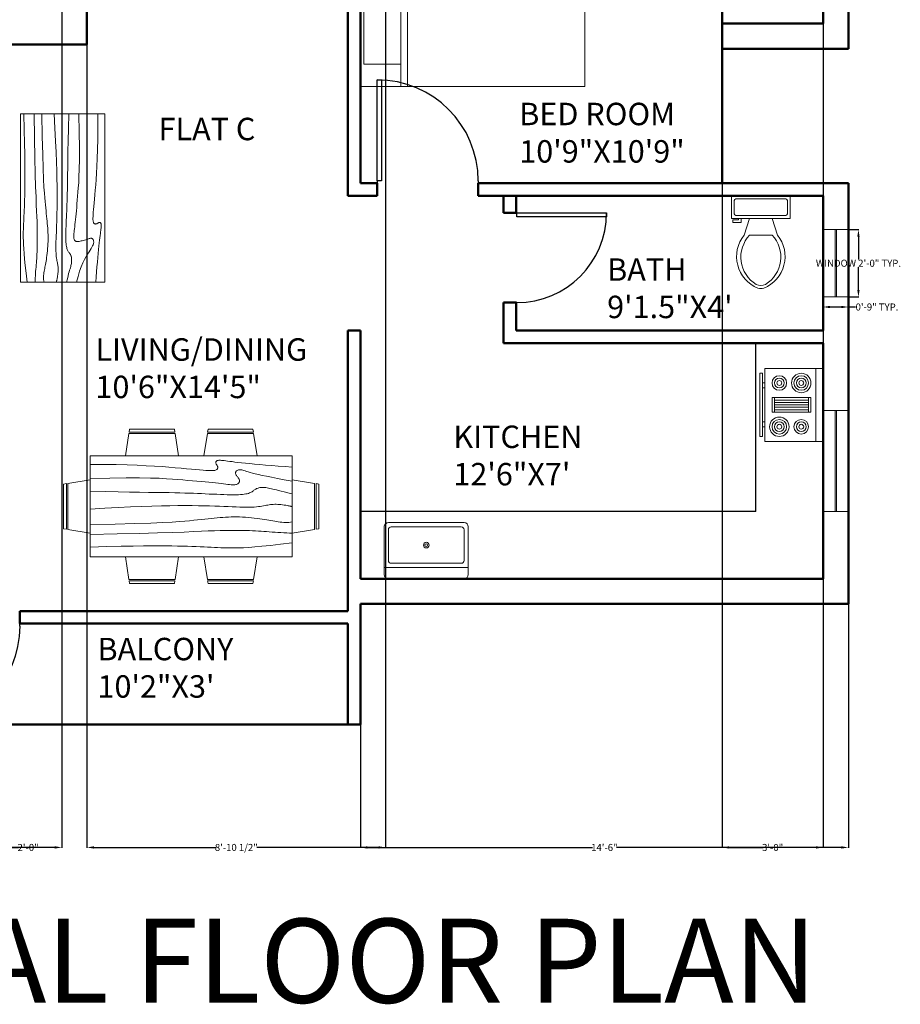
# Model space of a CAD drawing. Units: inches. Extents: x -46 to 565, y -56 to 809.
# Tile 2 of 6: x 221 to 535, y -56 to 296. Entities that reach past the tile are written whole.
import ezdxf

# ---------------------------------------------------------------- set-up
doc = ezdxf.new("R2010")
doc.units = ezdxf.units.IN
doc.header["$MEASUREMENT"] = 0
for name, color, linetype, lineweight in [('A-ANNO-DIMS', 2, 'Continuous', 18), ('A-ANNO-TEXT', 241, 'Continuous', 30), ('A-AREA-IDEN', 241, 'Continuous', 18), ('A-FLOR-CASE', 8, 'Continuous', 25), ('A-FLOR-FIXT', 131, 'Continuous', 18), ('A-FURN', 131, 'Continuous', 18), ('DOOR', 210, 'Continuous', 25), ('EQUIPMENT', 131, 'Continuous', 18), ('WALL', 10, 'Continuous', 50), ('WINDOW', 170, 'Continuous', 18)]:
    doc.layers.add(name, color=color, linetype=linetype, lineweight=lineweight)
doc.styles.get("Standard").update_dxf_attribs({"font": 'arial.ttf'})
doc.dimstyles.get("Standard").update_dxf_attribs({"dimtxt": 2.5, "dimasz": 2.5, "dimexe": 0.18, "dimexo": 0.0625, "dimgap": 0.09, "dimtad": 0, "dimtih": 1, "dimtoh": 1, "dimzin": 0, "dimdsep": 46, "dimlunit": 3, "dimtxsty": 'Standard', "dimcen": 0.09, "dimadec": 0, "dimazin": 0, "dimtfac": 1, "dimtofl": 0, "dimtmove": 0, "dimatfit": 3, "dimfxl": 1, "dimtolj": 1, "dimtzin": 0, "dimarcsym": 0})

# ---------------------------------------------------------------- blocks, each defined once
blk = doc.blocks.new('*U2')
for p, q in [((0, 0), (0, -6)), ((40, 0), (40, -6))]:
    blk.add_line(p, q)
blk.add_lwpolyline([(0, 0), (0, 40), (1.75, 40), (1.75, 0)], close=True)
blk.add_arc((0, 0), 40, 0, 90)
blk = doc.blocks.new('Bed - Queen')
for p, q in [((0, -80.00003), (0, 0)), ((0, 0), (59.99999, 0)), ((59.99999, 0), (59.99999, -80.00003)), ((7.99999, -1.2), (28.79998, -1.2)), ((7.99999, -14.4), (7.99999, -1.2)), ((28.79998, -1.2), (28.79998, -14.4)), ((31.19999, -1.2), (51.99999, -1.2)), ((31.19999, -14.4), (31.19999, -1.2)), ((51.99999, -1.2), (51.99999, -16.4)), ((0, -14.4), (44.8, -14.4)), ((44.8, -16.8), (0, -16.8)), ((59.99999, -29.6), (44.8, -14.4)), ((44.8, -14.4), (44.8, -29.6)), ((51.99999, -16.4), (46.79936, -16.4)), ((44.8, -29.6), (59.99999, -29.6)), ((59.99999, -80.00003), (0, -80.00003))]:
    blk.add_line(p, q)
blk = doc.blocks.new('Toilet - top')
for p, q in [((9.5, -6), (9.5, -2)), ((-10, -8.5), (-8, -8.5)), ((-10, -9.5), (-10, -8.5)), ((-7, -9.5), (-10, -9.5)), ((-8, -8.5), (-8, -8)), ((-7, -8), (-7, -9.5)), ((-4, -8), (-6, -14)), ((4, -8), (6, -14)), ((4, -14), (-4, -14))]:
    blk.add_line(p, q)
blk.add_lwpolyline([(10.5, -8), (10.5, 0), (-10.5, 0), (-10.5, -8)], close=True)
for points in [[(-9.5, -2), (-9.5, -6)], [(8.5, -1), (-8.5, -1)], [(-8.5, -7), (8.5, -7)]]:
    blk.add_lwpolyline(points)
for centre, radius, start, end in [((-8.62, -1.88), 0.884, 81.8699, 188.1301), ((8.62, -1.88), 0.884, 351.8699, 98.1301), ((-8.62, -6.12), 0.884, 171.8699, 278.1301), ((8.62, -6.12), 0.884, 261.8699, 8.1301), ((3.52, -21.58), 12.17, 141.4691, 247.9714), ((4.2, -21.82), 11.33, 136.3677, 238.9468), ((-3.52, -21.58), 12.17, 292.0284, 38.5307), ((-4.2, -21.82), 11.33, 301.053, 43.6321), ((0, -27.88), 4, 245.7318, 294.2682), ((0, -29), 4, 254.8605, 285.1395)]:
    blk.add_arc(centre, radius, start, end)
blk = doc.blocks.new('Dining Set - 36 x 72 in.')
for p, q in [((-22.2343, 26.00059), (-23.4847, 17.99762)), ((-22.2304, 26), (-5.7608, 26)), ((-22, 27.5), (-22.1562, 26.50042)), ((-5.8416, 26.5), (-22.1534, 26.5)), ((-22, 27.5), (-6, 27.5)), ((-5.8437, 26.49966), (-6, 27.5)), ((-4.5152, 17.99762), (-5.7655, 25.99926)), ((5.7657, 26.00059), (4.5153, 17.99762)), ((5.7696, 26), (22.2392, 26)), ((6, 27.5), (5.8438, 26.50042)), ((22.1584, 26.5), (5.8466, 26.5)), ((6, 27.5), (22, 27.5)), ((22.1563, 26.49966), (22, 27.5)), ((23.4848, 17.99762), (22.2345, 25.99926)), ((36, 18), (-36, 18)), ((-36, 18), (-36, -18)), ((36, -18), (36, 18)), ((-45.5, 8), (-44.5004, 8.15617)), ((-45.5, 8), (-45.5, -8)), ((-44.5, -8.15843), (-44.5, 8.15338)), ((-44.0006, 8.23428), (-35.9976, 9.48474)), ((-44, 8.23041), (-44, -8.23915)), ((44.0006, 8.23428), (35.9976, 9.48474)), ((44, 8.23041), (44, -8.23915)), ((44.5, -8.15843), (44.5, 8.15338)), ((45.5, 8), (44.5005, 8.15617)), ((45.5, 8), (45.5, -8)), ((-44.4997, -8.15631), (-45.5, -8)), ((-35.9976, -9.48476), (-43.9993, -8.2345)), ((35.9976, -9.48476), (43.9993, -8.2345)), ((44.4997, -8.15631), (45.5, -8)), ((-36, -18), (36, -18)), ((-22.2343, -26.0006), (-23.4847, -17.99762)), ((-4.5152, -17.99762), (-5.7655, -25.99928)), ((5.7657, -26.0006), (4.5153, -17.99762)), ((23.4848, -17.99762), (22.2345, -25.99928)), ((-22.2304, -26), (-5.7608, -26)), ((-22, -27.5), (-22.1562, -26.50044)), ((-5.8416, -26.5), (-22.1534, -26.5)), ((-22, -27.5), (-6, -27.5)), ((-5.8437, -26.49967), (-6, -27.5)), ((5.7696, -26), (22.2392, -26)), ((6, -27.5), (5.8438, -26.50044)), ((22.1584, -26.5), (5.8466, -26.5)), ((6, -27.5), (22, -27.5)), ((22.1563, -26.49967), (22, -27.5))]:
    blk.add_line(p, q)
for points in [[(-36, 15), (-31.1772, 14.97754), (-26.8079, 14.91406), (-22.8538, 14.81543), (-19.276, 14.6875), (-16.0362, 14.53613), (-13.0957, 14.36718), (-10.4159, 14.18652), (-7.9583, 14), (-5.6904, 13.81315), (-3.6035, 13.63021), (-1.6954, 13.45508), (0.0365, 13.29166), (1.5945, 13.14388), (2.9811, 13.01562), (4.1988, 12.9108), (5.25, 12.83333), (6.1393, 12.78613), (6.8802, 12.76823), (7.4883, 12.77767), (7.9792, 12.8125), (8.3685, 12.87077), (8.6719, 12.95052), (8.9049, 13.0498), (9.0833, 13.16666), (9.2205, 13.29899), (9.3216, 13.44401), (9.3895, 13.59879), (9.4271, 13.76041), (9.4373, 13.92594), (9.4232, 14.09245), (9.3875, 14.257), (9.3333, 14.41666), (9.2638, 14.56917), (9.1836, 14.71484), (9.0975, 14.85465), (9.0104, 14.98958), (8.9272, 15.1206), (8.8529, 15.2487), (8.7922, 15.37483), (8.75, 15.5), (8.7305, 15.62467), (8.7344, 15.74739), (8.7617, 15.86621), (8.8125, 15.97916), (8.8867, 16.08431), (8.9844, 16.17968), (9.1055, 16.26334), (9.25, 16.33333), (9.4189, 16.38802), (9.6172, 16.42708), (9.8506, 16.45052), (10.125, 16.45833), (10.4463, 16.45052), (10.8203, 16.42708), (11.2529, 16.38802), (11.75, 16.33333), (12.3184, 16.26318), (12.9694, 16.17838), (13.7151, 16.07991), (14.5677, 15.96875), (15.5395, 15.84586), (16.6426, 15.71224), (17.8893, 15.56884), (19.2917, 15.41666), (20.859, 15.25667), (22.5879, 15.08984), (24.4721, 14.91715), (26.5052, 14.73958), (28.6809, 14.5581), (30.9929, 14.3737), (33.4347, 14.18733), (36, 14)], [(-36, 10), (-28.9766, 10.14274), (-23.1725, 10.20442), (-18.4241, 10.19775), (-14.5677, 10.13541), (-11.4399, 10.03011), (-8.877, 9.89453), (-6.7154, 9.74137), (-4.7917, 9.58333), (-2.9698, 9.43082), (-1.2246, 9.28515), (0.4415, 9.14534), (2.026, 9.01041), (3.5266, 8.87939), (4.9408, 8.7513), (6.266, 8.62516), (7.5, 8.5), (8.6411, 8.37549), (9.6914, 8.2539), (10.6538, 8.13818), (11.5312, 8.03125), (12.3267, 7.93603), (13.043, 7.85547), (13.6831, 7.79248), (14.25, 7.75), (14.7471, 7.7303), (15.1797, 7.73307), (15.5537, 7.75732), (15.875, 7.80208), (16.1494, 7.86637), (16.3828, 7.94922), (16.5811, 8.04964), (16.75, 8.16666), (16.8944, 8.29915), (17.0143, 8.44531), (17.1089, 8.60319), (17.1771, 8.77083), (17.218, 8.94629), (17.2305, 9.1276), (17.2137, 9.31282), (17.1667, 9.5), (17.0895, 9.6875), (16.987, 9.875), (16.8649, 10.0625), (16.7292, 10.25), (16.5856, 10.4375), (16.4401, 10.625), (16.2985, 10.8125), (16.1667, 11), (16.05, 11.18733), (15.9518, 11.3737), (15.8752, 11.5581), (15.8229, 11.73958), (15.798, 11.91715), (15.8034, 12.08984), (15.842, 12.25667), (15.9167, 12.41666), (16.0295, 12.56836), (16.1784, 12.70833), (16.3605, 12.83268), (16.5729, 12.9375), (16.8127, 13.01888), (17.0768, 13.07291), (17.3625, 13.0957), (17.6667, 13.08333), (17.9894, 13.03312), (18.3418, 12.94726), (18.7382, 12.82918), (19.1927, 12.68229), (19.7195, 12.51001), (20.3327, 12.31575), (21.0465, 12.10294), (21.875, 11.875), (22.8357, 11.63354), (23.959, 11.37304), (25.2786, 11.08618), (26.8282, 10.76562), (28.6414, 10.40405), (30.752, 9.99414), (33.1936, 9.52856), (36, 9)], [(-36, 5.5), (-30.7157, 5.3348), (-26.069, 5.20963), (-21.9946, 5.11767), (-18.4271, 5.05208), (-15.3009, 5.00602), (-12.5508, 4.97265), (-10.1112, 4.94515), (-7.9167, 4.91666), (-5.909, 4.88167), (-4.0586, 4.83984), (-2.3429, 4.79215), (-0.7396, 4.73958), (0.7739, 4.6831), (2.22, 4.6237), (3.6213, 4.56233), (5, 4.5), (6.373, 4.43782), (7.7344, 4.3776), (9.0723, 4.32129), (10.375, 4.27083), (11.6309, 4.22819), (12.8281, 4.19531), (13.9551, 4.17415), (15, 4.16666), (15.954, 4.17448), (16.819, 4.19791), (17.6001, 4.23698), (18.3021, 4.29166), (18.9299, 4.36198), (19.4883, 4.44791), (19.9823, 4.54948), (20.4167, 4.66666), (20.7969, 4.79899), (21.1302, 4.94401), (21.4245, 5.09879), (21.6875, 5.26041), (21.9271, 5.42594), (22.1511, 5.59245), (22.3672, 5.757), (22.5834, 5.91666), (22.8065, 6.06868), (23.0404, 6.21093), (23.2879, 6.34147), (23.5521, 6.45833), (23.8358, 6.55957), (24.142, 6.64323), (24.4735, 6.70735), (24.8334, 6.75), (25.2235, 6.76969), (25.642, 6.76692), (26.0858, 6.74267), (26.5521, 6.69791), (27.0379, 6.63362), (27.5404, 6.55078), (28.0565, 6.45036), (28.5834, 6.33333), (29.1242, 6.19987), (29.7071, 6.04687), (30.3661, 5.87044), (31.1354, 5.66666), (32.0493, 5.43164), (33.142, 5.16146), (34.4475, 4.85221), (36, 4.5)], [(-36, -1), (-30.7915, -0.6591), (-26.0195, -0.38216), (-21.6519, -0.16284), (-17.6563, 0.00521), (-14.0005, 0.12833), (-10.6523, 0.21289), (-7.5796, 0.26522), (-4.75, 0.29166), (-2.134, 0.29793), (0.2878, 0.28711), (2.5317, 0.26163), (4.6146, 0.22396), (6.5529, 0.17651), (8.3633, 0.12174), (10.0623, 0.06209), (11.6667, 0), (13.1899, -0.06201), (14.6341, -0.1211), (15.9982, -0.17432), (17.2813, -0.21875), (18.4823, -0.25147), (19.6003, -0.26953), (20.6343, -0.27002), (21.5834, -0.25), (22.4481, -0.20768), (23.2357, -0.14584), (23.9549, -0.06836), (24.6146, 0.02083), (25.2235, 0.11784), (25.7904, 0.21875), (26.3241, 0.31966), (26.8334, 0.41666), (27.3265, 0.50618), (27.8099, 0.58593), (28.2894, 0.65397), (28.7709, 0.70833), (29.2601, 0.74707), (29.763, 0.76823), (30.2855, 0.76985), (30.8334, 0.75), (31.4088, 0.70784), (31.9994, 0.64713), (32.589, 0.57275), (33.1615, 0.48958), (33.7008, 0.4025), (34.1908, 0.3164), (34.6153, 0.23616), (34.9584, 0.16666), (35.2099, 0.11165), (35.3848, 0.07031), (35.504, 0.04069), (35.5886, 0.02083), (35.6594, 0.00879), (35.7377, 0.0026), (35.8442, 0.00032), (36, 0)], [(-36, -6.5), (-27.1843, -6.31267), (-20.084, -6.1263), (-14.469, -5.9419), (-10.1094, -5.76042), (-6.7752, -5.58285), (-4.2363, -5.41016), (-2.2629, -5.24333), (-0.625, -5.08334), (0.8708, -4.93099), (2.2715, -4.78646), (3.5872, -4.64974), (4.8281, -4.52084), (6.0046, -4.39974), (7.127, -4.28646), (8.2053, -4.18099), (9.25, -4.08334), (10.2705, -3.99382), (11.2734, -3.91407), (12.2647, -3.84603), (13.25, -3.79167), (14.2354, -3.75293), (15.2266, -3.73177), (16.2295, -3.73015), (17.25, -3.75), (18.2912, -3.79248), (19.3451, -3.85547), (20.4009, -3.93604), (21.4479, -4.03125), (22.4754, -4.13819), (23.4727, -4.25391), (24.4289, -4.37549), (25.3334, -4.5), (26.1785, -4.62492), (26.9694, -4.74935), (27.7145, -4.87281), (28.4219, -4.99479), (29.1, -5.11483), (29.7572, -5.23242), (30.4016, -5.34709), (31.0417, -5.45834), (31.6837, -5.56437), (32.3262, -5.65821), (32.9658, -5.73153), (33.599, -5.77604), (34.2224, -5.78345), (34.8327, -5.74545), (35.4264, -5.65373), (36, -5.5)], [(-36, -10), (-26.4022, -9.81299), (-18.4675, -9.62891), (-11.9839, -9.45069), (-6.7396, -9.28125), (-2.5226, -9.12354), (0.8789, -8.98047), (3.6769, -8.85498), (6.0833, -8.75), (8.2767, -8.66765), (10.3021, -8.60677), (12.1712, -8.56543), (13.8958, -8.54167), (15.4876, -8.53353), (16.9583, -8.53907), (18.3197, -8.55632), (19.5834, -8.58334), (20.7616, -8.61841), (21.8685, -8.66081), (22.9188, -8.71004), (23.9271, -8.76563), (24.9081, -8.82707), (25.8763, -8.89388), (26.8465, -8.96558), (27.8334, -9.04167), (28.8474, -9.12118), (29.8828, -9.20117), (30.93, -9.27824), (31.9792, -9.34896), (33.0205, -9.40991), (34.0443, -9.45768), (35.0407, -9.48885), (36, -9.5)], [(-36, -14.5), (-30.0881, -14.33513), (-25.0332, -14.21224), (-20.7312, -14.12647), (-17.0781, -14.07292), (-13.97, -14.04671), (-11.3027, -14.04297), (-8.9724, -14.05681), (-6.875, -14.08334), (-4.9224, -14.11833), (-3.0905, -14.16016), (-1.3709, -14.20785), (0.2448, -14.26042), (1.7647, -14.3169), (3.1973, -14.3763), (4.5507, -14.43767), (5.8333, -14.5), (7.0554, -14.5621), (8.235, -14.62175), (9.3922, -14.67652), (10.5469, -14.72396), (11.7192, -14.76164), (12.929, -14.78711), (14.1965, -14.79794), (15.5417, -14.79167), (16.9933, -14.76424), (18.6152, -14.70508), (20.4804, -14.60197), (22.6615, -14.44271), (25.2312, -14.21509), (28.2624, -13.9069), (31.8277, -13.50594), (36, -13)]]:
    blk.add_lwpolyline(points)
blk = doc.blocks.new('Table - Rectangular Woodgrain 60 x 30 in.')
for p, q in [((0, 0), (0, -30)), ((60, 0), (0, 0)), ((60, -30), (60, 0)), ((0, -30), (60, -30))]:
    blk.add_line(p, q)
for points in [[(0, -2.4), (4.8155, -2.418), (9.0302, -2.4688), (12.709, -2.5477), (15.9167, -2.65), (18.7181, -2.7711), (21.1781, -2.9063), (23.3616, -3.0508), (25.3333, -3.2), (27.1477, -3.3495), (28.8172, -3.4958), (30.3437, -3.636), (31.7291, -3.7667), (32.9756, -3.8849), (34.0849, -3.9875), (35.059, -4.0714), (35.9, -4.1334), (36.6114, -4.1711), (37.2041, -4.1854), (37.6906, -4.1779), (38.0833, -4.15), (38.3948, -4.1034), (38.6375, -4.0396), (38.8239, -3.9602), (38.9666, -3.8667), (39.0764, -3.7608), (39.1573, -3.6448), (39.2116, -3.521), (39.2416, -3.3917), (39.2498, -3.2593), (39.2385, -3.1261), (39.21, -2.9944), (39.1666, -2.8667), (39.111, -2.7447), (39.0468, -2.6281), (38.978, -2.5163), (38.9083, -2.4083), (38.8418, -2.3035), (38.7823, -2.201), (38.7337, -2.1001), (38.7, -2), (38.6844, -1.9003), (38.6875, -1.8021), (38.7094, -1.707), (38.75, -1.6167), (38.8094, -1.5326), (38.8875, -1.4563), (38.9844, -1.3893), (39.1, -1.3333), (39.2351, -1.2896), (39.3937, -1.2583), (39.5804, -1.2396), (39.8, -1.2333), (40.057, -1.2396), (40.3562, -1.2583), (40.7023, -1.2896), (41.1, -1.3333), (41.5547, -1.3895), (42.0755, -1.4573), (42.6721, -1.5361), (43.3542, -1.625), (44.1316, -1.7233), (45.014, -1.8302), (46.0114, -1.9449), (47.1333, -2.0667), (48.3862, -2.1947), (49.7625, -2.3281), (51.2513, -2.4663), (52.8416, -2.6083), (54.5226, -2.7535), (56.2833, -2.9011), (58.1127, -3.0501), (60, -3.2)], [(0, -9.2), (6.5759, -9.0858), (11.9385, -9.0365), (16.2527, -9.0418), (19.6833, -9.0917), (22.3952, -9.1759), (24.5531, -9.2844), (26.322, -9.4069), (27.8666, -9.5333), (29.3241, -9.6553), (30.7203, -9.7719), (32.0532, -9.8837), (33.3208, -9.9917), (34.5213, -10.0965), (35.6526, -10.199), (36.7128, -10.2999), (37.7, -10.4), (38.6129, -10.4996), (39.4531, -10.5969), (40.223, -10.6895), (40.925, -10.775), (41.5613, -10.8512), (42.1344, -10.9156), (42.6465, -10.966), (43.1, -11), (43.4976, -11.0158), (43.8437, -11.0136), (44.143, -10.9942), (44.4, -10.9583), (44.6195, -10.9069), (44.8062, -10.8406), (44.9648, -10.7603), (45.1, -10.6667), (45.2155, -10.5598), (45.3114, -10.4365), (45.3871, -10.2929), (45.4416, -10.125), (45.4743, -9.929), (45.4844, -9.7011), (45.4709, -9.4371), (45.4333, -9.1333), (45.3716, -8.7883), (45.2896, -8.4104), (45.1919, -8.0107), (45.0833, -7.6), (44.9685, -7.1893), (44.8521, -6.7896), (44.7388, -6.4117), (44.6333, -6.0667), (44.54, -5.7628), (44.4614, -5.4979), (44.4001, -5.2675), (44.3583, -5.0667), (44.3384, -4.8909), (44.3427, -4.7354), (44.3736, -4.5956), (44.4333, -4.4667), (44.5236, -4.3453), (44.6427, -4.2333), (44.7884, -4.1339), (44.9583, -4.05), (45.1501, -3.9849), (45.3614, -3.9417), (45.59, -3.9234), (45.8333, -3.9333), (46.0915, -3.9749), (46.3734, -4.0531), (46.6906, -4.1736), (47.0542, -4.3417), (47.4756, -4.5629), (47.9661, -4.8427), (48.5372, -5.1866), (49.2, -5.6), (49.9676, -6.0844), (50.8594, -6.625), (51.8965, -7.2031), (53.1, -7.8), (54.491, -8.3969), (56.0906, -8.975), (57.9199, -9.5156), (60, -10)], [(0, -12.8), (5.1847, -12.9322), (9.6213, -13.0323), (13.3963, -13.1059), (16.5958, -13.1583), (19.3063, -13.1952), (21.614, -13.2219), (23.6054, -13.2439), (25.3666, -13.2667), (26.9728, -13.2947), (28.4531, -13.3281), (29.8256, -13.3663), (31.1083, -13.4083), (32.3191, -13.4535), (33.476, -13.501), (34.597, -13.5501), (35.7, -13.6), (36.7984, -13.6497), (37.8875, -13.6979), (38.9578, -13.743), (40, -13.7833), (41.0047, -13.8174), (41.9625, -13.8438), (42.864, -13.8607), (43.7, -13.8667), (44.4631, -13.8604), (45.1552, -13.8417), (45.7801, -13.8104), (46.3416, -13.7667), (46.8439, -13.7104), (47.2906, -13.6417), (47.6858, -13.5604), (48.0333, -13.4667), (48.3375, -13.3608), (48.6042, -13.2448), (48.8396, -13.121), (49.05, -12.9917), (49.2417, -12.8593), (49.4208, -12.7261), (49.5937, -12.5944), (49.7667, -12.4667), (49.9452, -12.3451), (50.1323, -12.2313), (50.3303, -12.1268), (50.5416, -12.0333), (50.7686, -11.9524), (51.0135, -11.8854), (51.2788, -11.8341), (51.5666, -11.8), (51.8785, -11.7843), (52.2116, -11.7865), (52.562, -11.8059), (52.926, -11.8417), (53.2998, -11.8931), (53.6795, -11.9594), (54.0614, -12.0397), (54.4416, -12.1333), (54.8223, -12.2401), (55.2293, -12.3625), (55.6942, -12.5037), (56.2489, -12.6667), (56.9251, -12.8547), (57.7545, -13.0708), (58.7689, -13.3182), (60, -13.6)], [(0, -18), (5.124, -17.7273), (9.6609, -17.5057), (13.6705, -17.3303), (17.2125, -17.1958), (20.3467, -17.0973), (23.1328, -17.0297), (25.6307, -16.9878), (27.9, -16.9667), (29.9928, -16.9617), (31.9302, -16.9703), (33.7254, -16.9907), (35.3917, -17.0208), (36.9423, -17.0588), (38.3906, -17.1026), (39.7499, -17.1503), (41.0333, -17.2), (42.2519, -17.2496), (43.4073, -17.2969), (44.4986, -17.3395), (45.525, -17.375), (46.4858, -17.4012), (47.3802, -17.4156), (48.2074, -17.416), (48.9667, -17.4), (49.6583, -17.3662), (50.2872, -17.3167), (50.8595, -17.2547), (51.3812, -17.1833), (51.8584, -17.1057), (52.2971, -17.025), (52.7034, -16.9443), (53.0833, -16.8667), (53.443, -16.7951), (53.789, -16.7313), (54.128, -16.6768), (54.4666, -16.6334), (54.8115, -16.6024), (55.1693, -16.5854), (55.5465, -16.5841), (55.95, -16.6), (56.3828, -16.6337), (56.8346, -16.6823), (57.2915, -16.7418), (57.7396, -16.8084), (58.165, -16.878), (58.5539, -16.9469), (58.8924, -17.0111), (59.1666, -17.0667), (59.3679, -17.1107), (59.5078, -17.1438), (59.6032, -17.1675), (59.6708, -17.1833), (59.7275, -17.193), (59.7901, -17.1979), (59.8753, -17.1998), (60, -17.2)], [(0, -22.4), (8.0098, -22.2501), (14.4094, -22.1011), (19.4168, -21.9535), (23.25, -21.8083), (26.1269, -21.6663), (28.2656, -21.5281), (29.884, -21.3947), (31.2, -21.2667), (32.3967, -21.1448), (33.5172, -21.0292), (34.5697, -20.9198), (35.5625, -20.8167), (36.5037, -20.7198), (37.4015, -20.6292), (38.2642, -20.5448), (39.1, -20.4667), (39.9164, -20.3951), (40.7187, -20.3313), (41.5117, -20.2768), (42.3, -20.2333), (43.0883, -20.2024), (43.8812, -20.1854), (44.6836, -20.1841), (45.5, -20.2), (46.3328, -20.234), (47.1747, -20.2844), (48.0163, -20.3488), (48.8479, -20.425), (49.66, -20.5106), (50.4429, -20.6031), (51.1872, -20.7004), (51.8833, -20.8), (52.5246, -20.8999), (53.1166, -20.9995), (53.6681, -21.0983), (54.1875, -21.1958), (54.6834, -21.2919), (55.1646, -21.3859), (55.6394, -21.4777), (56.1167, -21.5667), (56.6028, -21.6515), (57.0961, -21.7266), (57.5929, -21.7852), (58.0896, -21.8208), (58.5823, -21.8268), (59.0674, -21.7964), (59.5412, -21.723), (60, -21.6)], [(0, -25.2), (8.6355, -25.0504), (15.7026, -24.9031), (21.4049, -24.7606), (25.9458, -24.625), (29.529, -24.4988), (32.3578, -24.3844), (34.6359, -24.284), (36.5667, -24.2), (38.3213, -24.1341), (39.9417, -24.0854), (41.437, -24.0523), (42.8167, -24.0333), (44.0901, -24.0268), (45.2667, -24.0313), (46.3557, -24.0451), (47.3667, -24.0667), (48.309, -24.0947), (49.1928, -24.1287), (50.0284, -24.168), (50.826, -24.2125), (51.5959, -24.2617), (52.3483, -24.3151), (53.0935, -24.3725), (53.8417, -24.4334), (54.6009, -24.497), (55.3699, -24.561), (56.1454, -24.6226), (56.9239, -24.6792), (57.7021, -24.7279), (58.4764, -24.7662), (59.2435, -24.7911), (60, -24.8)], [(0, -28.8), (5.6867, -28.6681), (10.45, -28.5698), (14.407, -28.5012), (17.675, -28.4584), (20.3711, -28.4374), (22.6125, -28.4344), (24.5164, -28.4455), (26.2, -28.4667), (27.762, -28.4947), (29.2276, -28.5281), (30.6033, -28.5663), (31.8958, -28.6084), (33.1118, -28.6535), (34.2578, -28.7011), (35.3405, -28.7501), (36.3666, -28.8), (37.3443, -28.8497), (38.288, -28.8974), (39.2137, -28.9412), (40.1375, -28.9792), (41.0753, -29.0093), (42.0432, -29.0297), (43.0572, -29.0384), (44.1333, -29.0333), (45.2936, -29.0114), (46.5843, -28.9641), (48.0579, -28.8816), (49.7666, -28.7542), (51.7629, -28.5721), (54.0989, -28.3255), (56.8272, -28.0048), (60, -27.6)]]:
    blk.add_lwpolyline(points)
blk = doc.blocks.new('Range-Oven - 30 in top')
for p, q in [((0, -3), (30, -3)), ((12, -6), (18, -6)), ((13, -20), (13, -6)), ((14, -6), (14, -20)), ((15, -20), (15, -6)), ((16, -6), (16, -20)), ((17, -20), (17, -6)), ((18, -20), (12, -20)), ((6, -24), (6, -25)), ((8, -25), (8, -24)), ((22, -25), (22, -24)), ((24, -24), (24, -25))]:
    blk.add_line(p, q)
for points in [[(0, -24), (0, 0), (30, 0), (30, -24)], [(12, -21), (12, -5), (18, -5), (18, -21)], [(2, -26), (2, -25), (28, -25), (28, -26)]]:
    blk.add_lwpolyline(points, close=True)
for centre, radius in [((6, -9), 4), ((6, -9), 3), ((6, -9), 2), ((6, -9), 1), ((24, -9), 3), ((24, -9), 2), ((24, -9), 1), ((6, -18), 3), ((6, -18), 2), ((24, -18), 4), ((24, -18), 3), ((24, -18), 2), ((6, -18), 1), ((24, -18), 1)]:
    blk.add_circle(centre, radius)
blk = doc.blocks.new('Sink-single - 30 in top')
blk.add_line((-15, -3.999996), (15, -3.999996))
for points in [[(-13.5, 0), (13.5, 0)], [(-15, -18.499996), (-15, -1.5)], [(15, -1.5), (15, -18.499996)], [(-13.5, -17.499996), (-13.5, -6.499996)], [(-12.5, -5.499996), (12.5, -5.499996)], [(13.5, -6.499996), (13.5, -17.499996)], [(13.5, -19.999996), (-13.5, -19.999996)], [(12.5, -18.499996), (-12.5, -18.499996)]]:
    blk.add_lwpolyline(points)
for radius in [1, 0.5]:
    blk.add_circle((0, -11.999996), radius)
for centre, radius, start, end in [((-13.5, -1.5), 1.5, 90, 180), ((13.5, -1.5), 1.5, 0, 90), ((-12.5, -6.499996), 1, 90, 180), ((12.5, -6.499996), 1, 0, 90), ((-12.5, -17.499996), 1, 180, 270), ((12.5, -17.499996), 1, 270, 0), ((-13.5, -18.499996), 1.5, 180, 270), ((13.5, -18.499996), 1.5, 270, 0)]:
    blk.add_arc(centre, radius, start, end)
blk = doc.blocks.new('WIN-24IN')
for p, q in [((4.25, 24), (4.25, 0)), ((4.75, 24), (4.75, 0))]:
    blk.add_line(p, q)
blk.add_lwpolyline([(0, 24), (0, 0), (9, 0), (9, 24)], close=True)
blk = doc.blocks.new('WIN-36IN')
for p, q in [((4.25, 36), (4.25, 0)), ((4.75, 36), (4.75, 0))]:
    blk.add_line(p, q)
blk.add_lwpolyline([(0, 36), (0, 0), (9, 0), (9, 36)], close=True)
blk = doc.blocks.new('*D25')
at = {"layer": 'A-ANNO-DIMS', "color": 0, "lineweight": -2, "transparency": 16777216}
for p, q in [((516.21, 220.7), (519.92, 220.7)), ((519.74, 218.2), (519.74, 210.08)), ((519.74, 199.2), (519.74, 207.32)), ((516.21, 196.7), (519.92, 196.7))]:
    blk.add_line(p, q, dxfattribs=at)
at = {"layer": 'A-ANNO-DIMS', "color": 0, "transparency": 16777216}
for points in [[(519.33, 218.2), (520.16, 218.2), (519.74, 220.7)], [(519.33, 199.2), (520.16, 199.2), (519.74, 196.7)]]:
    blk.add_solid(points, dxfattribs=at)
at = {"layer": 'Defpoints', "color": 0, "transparency": 16777216}
for p in [(516.14, 220.7), (519.74, 220.7), (516.14, 196.7)]:
    blk.add_point(p, dxfattribs=at)
at = {"layer": 'A-ANNO-DIMS', "color": 0, "transparency": 16777216, "insert": (519.74, 208.7), "char_height": 2.5, "attachment_point": 5}
blk.add_mtext('\\A1;WINDOW 2\'-0" TYP.', dxfattribs=at)
blk = doc.blocks.new('*D26')
at = {"layer": 'A-ANNO-DIMS', "color": 0, "lineweight": -2, "transparency": 16777216}
for p, q in [((507.14, 196.64), (507.14, 192.92)), ((516.14, 196.64), (516.14, 192.92)), ((509.64, 193.1), (513.64, 193.1)), ((516.14, 193.1), (518.64, 193.1))]:
    blk.add_line(p, q, dxfattribs=at)
at = {"layer": 'A-ANNO-DIMS', "color": 0, "transparency": 16777216}
for points in [[(509.64, 193.52), (509.64, 192.68), (507.14, 193.1)], [(513.64, 193.52), (513.64, 192.68), (516.14, 193.1)]]:
    blk.add_solid(points, dxfattribs=at)
at = {"layer": 'Defpoints', "color": 0, "transparency": 16777216}
for p in [(507.14, 196.7), (516.14, 196.7), (516.14, 193.1)]:
    blk.add_point(p, dxfattribs=at)
at = {"layer": 'A-ANNO-DIMS', "color": 0, "transparency": 16777216, "insert": (526.35, 193.1), "char_height": 2.5, "attachment_point": 5}
blk.add_mtext('\\A1;0\'-9" TYP.', dxfattribs=at)
blk = doc.blocks.new('*D42')
at = {"layer": 'A-ANNO-DIMS', "color": 0, "lineweight": -2, "transparency": 16777216}
for p, q in [((471.14, 375.14), (471.14, 0.22)), ((507.14, 375.14), (507.14, 0.22)), ((473.64, 0.4), (485.73, 0.4)), ((504.64, 0.4), (492.55, 0.4))]:
    blk.add_line(p, q, dxfattribs=at)
at = {"layer": 'A-ANNO-DIMS', "color": 0, "transparency": 16777216}
for points in [[(473.64, 0.82), (473.64, -0.02), (471.14, 0.4)], [(504.64, 0.82), (504.64, -0.02), (507.14, 0.4)]]:
    blk.add_solid(points, dxfattribs=at)
at = {"layer": 'Defpoints', "color": 0, "transparency": 16777216}
for p in [(471.14, 375.2), (507.14, 375.2), (507.14, 0.4)]:
    blk.add_point(p, dxfattribs=at)
at = {"layer": 'A-ANNO-DIMS', "color": 0, "transparency": 16777216, "insert": (489.14, 0.4), "char_height": 2.5, "attachment_point": 5}
blk.add_mtext('\\A1;3\'-0"', dxfattribs=at)
blk = doc.blocks.new('*D43')
at = {"layer": 'A-ANNO-DIMS', "color": 0, "lineweight": -2, "transparency": 16777216}
for p, q in [((244.64, 375.14), (244.64, 0.22)), ((351.14, 375.14), (351.14, 0.22)), ((247.14, 0.4), (290.59, 0.4)), ((348.64, 0.4), (305.19, 0.4))]:
    blk.add_line(p, q, dxfattribs=at)
at = {"layer": 'A-ANNO-DIMS', "color": 0, "transparency": 16777216}
for points in [[(247.14, 0.82), (247.14, -0.02), (244.64, 0.4)], [(348.64, 0.82), (348.64, -0.02), (351.14, 0.4)]]:
    blk.add_solid(points, dxfattribs=at)
at = {"layer": 'Defpoints', "color": 0, "transparency": 16777216}
for p in [(244.64, 375.2), (351.14, 375.2), (351.14, 0.4)]:
    blk.add_point(p, dxfattribs=at)
at = {"layer": 'A-ANNO-DIMS', "color": 0, "transparency": 16777216, "insert": (297.89, 0.4), "char_height": 2.5, "attachment_point": 5}
blk.add_mtext('\\A1;8\'-10 1/2"', dxfattribs=at)
blk = doc.blocks.new('*D49')
at = {"layer": 'A-ANNO-DIMS', "color": 0, "lineweight": -2, "transparency": 16777216}
for p, q in [((516.14, 87.14), (516.14, 0.22)), ((342.14, 44.14), (342.14, 0.22)), ((344.64, 0.4), (424.88, 0.4)), ((513.64, 0.4), (433.41, 0.4))]:
    blk.add_line(p, q, dxfattribs=at)
at = {"layer": 'A-ANNO-DIMS', "color": 0, "transparency": 16777216}
for points in [[(344.64, 0.82), (344.64, -0.02), (342.14, 0.4)], [(513.64, 0.82), (513.64, -0.02), (516.14, 0.4)]]:
    blk.add_solid(points, dxfattribs=at)
at = {"layer": 'Defpoints', "color": 0, "transparency": 16777216}
for p in [(516.14, 87.2), (342.14, 44.2), (516.14, 0.4)]:
    blk.add_point(p, dxfattribs=at)
at = {"layer": 'A-ANNO-DIMS', "color": 0, "transparency": 16777216, "insert": (429.14, 0.4), "char_height": 2.5, "attachment_point": 5}
blk.add_mtext('\\A1;14\'-6"', dxfattribs=at)
blk = doc.blocks.new('*D50')
at = {"layer": 'A-ANNO-DIMS', "color": 0, "lineweight": -2, "transparency": 16777216}
for p, q in [((211.64, 558.64), (211.64, 0.22)), ((235.64, 558.64), (235.64, 0.22)), ((214.14, 0.4), (220.21, 0.4)), ((233.14, 0.4), (227.08, 0.4))]:
    blk.add_line(p, q, dxfattribs=at)
at = {"layer": 'A-ANNO-DIMS', "color": 0, "transparency": 16777216}
for points in [[(214.14, 0.82), (214.14, -0.02), (211.64, 0.4)], [(233.14, 0.82), (233.14, -0.02), (235.64, 0.4)]]:
    blk.add_solid(points, dxfattribs=at)
at = {"layer": 'Defpoints', "color": 0, "transparency": 16777216}
for p in [(211.64, 558.7), (235.64, 558.7), (235.64, 0.4)]:
    blk.add_point(p, dxfattribs=at)
at = {"layer": 'A-ANNO-DIMS', "color": 0, "transparency": 16777216, "insert": (223.64, 0.4), "char_height": 2.5, "attachment_point": 5}
blk.add_mtext('\\A1;2\'-0"', dxfattribs=at)
blk = doc.blocks.new('*D55')
at = {"layer": 'A-ANNO-DIMS', "color": 0, "lineweight": -2, "transparency": 16777216}
for p, q in [((45.14, 407.14), (45.14, 0.22)), ((235.64, 407.14), (235.64, 0.22)), ((47.64, 0.4), (132.24, 0.4)), ((233.14, 0.4), (148.54, 0.4))]:
    blk.add_line(p, q, dxfattribs=at)
at = {"layer": 'A-ANNO-DIMS', "color": 0, "transparency": 16777216}
for points in [[(47.64, 0.82), (47.64, -0.02), (45.14, 0.4)], [(233.14, 0.82), (233.14, -0.02), (235.64, 0.4)]]:
    blk.add_solid(points, dxfattribs=at)
at = {"layer": 'Defpoints', "color": 0, "transparency": 16777216}
for p in [(45.14, 407.2), (235.64, 407.2), (235.64, 0.4)]:
    blk.add_point(p, dxfattribs=at)
at = {"layer": 'A-ANNO-DIMS', "color": 0, "transparency": 16777216, "insert": (140.39, 0.4), "char_height": 2.5, "attachment_point": 5}
blk.add_mtext('\\A1;15\'-10 1/2"', dxfattribs=at)

msp = doc.modelspace()

# ---------------------------------------------------------------- linework, layer by layer
at = {"layer": 'A-FLOR-CASE'}
for q in [(483.143, 180.2), (342.143, 120.2)]:
    msp.add_line((483.143, 120.2), q, dxfattribs=at)
at = {"layer": 'WALL'}
for p, q in [((516.143, 285.2), (516.143, 462.2)), ((507.143, 294.2), (507.143, 375.2)), ((244.643, 366.2), (244.643, 286.7)), ((337.643, 232.7), (337.643, 366.2)), ((342.143, 237.2), (342.143, 366.2)), ((471.143, 237.2), (471.143, 366.2)), ((507.143, 294.2), (471.143, 294.2)), ((244.643, 286.7), (178.643, 286.7)), ((516.143, 285.2), (471.143, 285.2)), ((348.143, 237.2), (342.143, 237.2)), ((348.143, 237.2), (348.143, 232.7)), ((516.143, 237.2), (384.143, 237.2)), ((384.143, 237.2), (384.143, 232.7)), ((516.143, 87.2), (516.143, 237.2)), ((348.143, 232.7), (337.643, 232.7)), ((393.143, 232.7), (384.143, 232.7)), ((393.143, 232.7), (397.643, 232.7)), ((393.143, 226.7), (393.143, 232.7)), ((507.143, 232.7), (397.643, 232.7)), ((397.643, 226.7), (397.643, 232.7)), ((507.143, 184.7), (507.143, 232.7)), ((393.143, 226.7), (397.643, 226.7)), ((393.143, 180.2), (393.143, 194.7)), ((393.143, 194.7), (397.643, 194.7)), ((397.643, 184.7), (397.643, 194.7)), ((337.643, 87.2), (337.643, 184.7)), ((342.143, 184.7), (337.643, 184.7)), ((342.143, 96.2), (342.143, 184.7)), ((393.143, 184.7), (393.143, 180.2)), ((507.143, 184.7), (397.643, 184.7)), ((507.143, 180.2), (393.143, 180.2)), ((507.143, 96.2), (507.143, 180.2)), ((507.143, 96.2), (342.143, 96.2)), ((337.643, 84.7), (220.643, 84.7)), ((220.643, 84.7), (220.643, 80.2)), ((244.643, 84.7), (337.643, 84.7)), ((337.643, 87.2), (337.643, 84.7)), ((342.143, 53.2), (342.143, 87.2)), ((516.143, 87.2), (342.143, 87.2)), ((337.643, 80.2), (220.643, 80.2)), ((244.643, 80.2), (337.643, 80.2)), ((337.643, 80.2), (337.643, 44.2)), ((342.143, 44.2), (342.143, 53.2)), ((235.643, 44.2), (174.143, 44.2)), ((235.643, 44.2), (244.643, 44.2)), ((244.643, 44.2), (342.143, 44.2))]:
    msp.add_line(p, q, dxfattribs=at)

# ---------------------------------------------------------------- block references
at = {"layer": 'A-FLOR-FIXT'}
msp.add_blockref('Toilet - top', (484.935, 232.7), dxfattribs=at)
at = {"layer": 'A-FLOR-FIXT', "rotation": 180}
msp.add_blockref('Sink-single - 30 in top', (365.627, 96.2), dxfattribs=at)
at = {"layer": 'A-FURN'}
for name, p, rotation in [('Bed - Queen', (342.143, 271.7), 90), ('Table - Rectangular Woodgrain 60 x 30 in.', (250.96, 261.941), 270)]:
    msp.add_blockref(name, p, dxfattribs=dict(at, rotation=rotation))
msp.add_blockref('Dining Set - 36 x 72 in.', (281.818, 121.983), dxfattribs=at)
at = {"layer": 'DOOR', "xscale": 0.9, "yscale": 0.9, "zscale": 0.9}
msp.add_blockref('*U2', (348.143, 238.1), dxfattribs=at)
at = {"layer": 'DOOR'}
for p, xscale, yscale, zscale, rotation in [((397.943, 226.7), 0.7999999999999993, 0.7999999999999993, 0.7999999999999993, 270), ((184.643, 79.3), -0.8999999999999971, 0.8999999999999971, 0.8999999999999971, 180)]:
    msp.add_blockref('*U2', p, dxfattribs=dict(at, xscale=xscale, yscale=yscale, zscale=zscale, rotation=rotation))
at = {"layer": 'EQUIPMENT', "xscale": 0.8666666666666667, "yscale": 0.8666666666666667, "zscale": 0.8666666666666667, "rotation": 270}
msp.add_blockref('Range-Oven - 30 in top', (507.143, 171.2), dxfattribs=at)
at = {"layer": 'WINDOW'}
for name, p in [('WIN-24IN', (507.143, 196.7)), ('WIN-36IN', (507.143, 120.2))]:
    msp.add_blockref(name, p, dxfattribs=at)

# ---------------------------------------------------------------- texts
at = {"layer": 'A-ANNO-TEXT', "insert": (0.465, -25.004), "char_height": 30, "attachment_point": 1}
msp.add_mtext_dynamic_manual_height_columns('RESIDENTIAL FLOOR PLAN', width=551.91415, gutter_width=1, heights=[0], dxfattribs=at)
at = {"layer": 'A-AREA-IDEN', "char_height": 8, "attachment_point": 1}
for s, insert in [('BED ROOM\\P10\'9"X10\'9" ', (398.782, 265.92)), ('FLAT C', (270.158, 260.567)), ('BATH\\P9\'1.5"X4\'', (430.12, 210.458)), ('LIVING/DINING\\P10\'6"X14\'5" ', (247.657, 181.937)), ('KITCHEN\\P12\'6"X7\' ', (375.293, 150.821)), ('BALCONY\\P10\'2"X3\' ', (248.38, 75.135))]:
    msp.add_mtext_dynamic_manual_height_columns(s, width=70.77133, gutter_width=1, heights=[0], dxfattribs=dict(at, insert=insert))

# ---------------------------------------------------------------- dimensions: what is measured, and where the dimension line sits
at = {"layer": 'A-ANNO-DIMS'}
for base, p1, p2, picture, middle in [((235.643, 0.4), (211.643, 558.7), (235.643, 558.7), '*D50', (223.643, 0.4)), ((235.643, 0.4), (45.143, 407.2), (235.643, 407.2), '*D55', (140.393, 0.4)), ((351.143, 0.4), (244.643, 375.2), (351.143, 375.2), '*D43', (297.893, 0.4)), ((507.143, 0.4), (471.143, 375.2), (507.143, 375.2), '*D42', (489.143, 0.4)), ((516.143, 0.4), (342.143, 44.2), (516.143, 87.2), '*D49', (429.143, 0.4))]:
    dim = msp.add_linear_dim(base=base, p1=p1, p2=p2, dimstyle='Standard', override={"dimdec": 1, "dimlfac": 1, "dimrnd": 0, "dimzin": 1, "dimdsep": 46, "dimlunit": 4, "dimfrac": 2}, dxfattribs=at)
    dim.commit()
    dim.dimension.update_dxf_attribs({"geometry": picture, "text_midpoint": middle})
dim = msp.add_linear_dim(base=(519.743, 220.7), p1=(516.143, 196.7), p2=(516.143, 220.7), angle=90, text='WINDOW <> TYP.', dimstyle='Standard', override={"dimdec": 1, "dimlfac": 1, "dimrnd": 0, "dimzin": 1, "dimdsep": 46, "dimlunit": 4, "dimfrac": 2}, dxfattribs=at)
dim.commit()
dim.dimension.update_dxf_attribs({"geometry": '*D25', "text_midpoint": (519.743, 208.7)})
dim = msp.add_linear_dim(base=(516.143, 193.1), p1=(507.143, 196.7), p2=(516.143, 196.7), text='<> TYP.', dimstyle='Standard', override={"dimdec": 1, "dimlfac": 1, "dimrnd": 0, "dimzin": 1, "dimdsep": 46, "dimlunit": 4, "dimfrac": 2}, dxfattribs=at)
dim.commit()
dim.dimension.update_dxf_attribs({"geometry": '*D26', "text_midpoint": (526.352, 193.1)})

doc.saveas('drawing.dxf')
